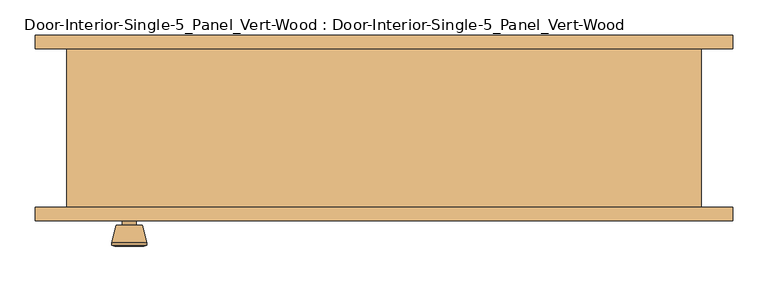
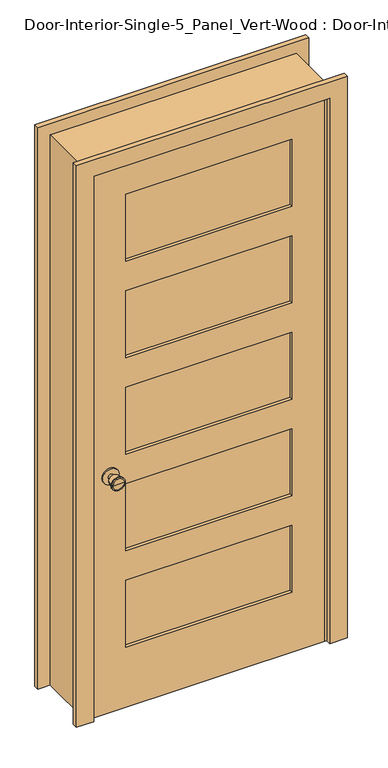
"""IFC4 building model written with IfcOpenShell, lengths in millimetres: door geometry, Door-Interior-Single-5_Panel_Vert-Wood : Door-Interior-Single-5_Panel_Vert-Wood."""

from ifc_helpers import new_model, si_unit, point, frame, frame_2d, origin, place, context, project, spatial, polyline, circle_curve, trimmed, segment, composite_curve, outline, extrude, faceted_brep, source, transform, mapped, element, save
from ifc_brep_helpers import plane_surface, cylinder_surface, revolved_surface, advanced_brep


def door_interior_single_5_panel_vert_wood_door_interior_single_643f6a0b(model_context):
    return source(origin(), model_context, "Body", "SolidModel", [
        advanced_brep(
        [(-361.1, -68.4, 914.4), (-371.1, -68.4, 914.4), (-351.1, -68.4, 914.4), (-340.6241324, -19.4, 914.4), (-381.5758676, -19.4, 914.4), (-361.1, -19.4, 914.4), (-336.1, -21.2278681, 914.4), (-386.1, -21.2278681, 914.4), (-336.1, -24.6915463, 914.4), (-386.1, -24.6915463, 914.4), (-342.463764, -49.4, 914.4), (-379.736236, -49.4, 914.4), (-351.1, -49.4, 914.4), (-371.1, -49.4, 914.4)],
        [
            (0, 1),
            (1, 2, circle_curve(frame((-361.1, -68.4, 914.4), z_axis=(0.0, -1.0, 0.0), x_axis=(-1.0, 0.0, 0.0)), 10.0)),
            (2, 0),
            (2, 1, circle_curve(frame((-361.1, -68.4, 914.4), z_axis=(0.0, -1.0, 0.0), x_axis=(-1.0, 0.0, 0.0)), 10.0)),
            (3, 4, circle_curve(frame((-361.1, -19.4, 914.4), z_axis=(0.0, 1.0, 0.0), x_axis=(-1.0, 0.0, 0.0)), 20.4758676)),
            (4, 5),
            (5, 3),
            (4, 3, circle_curve(frame((-361.1, -19.4, 914.4), z_axis=(0.0, 1.0, 0.0), x_axis=(-1.0, 0.0, 0.0)), 20.4758676)),
            (6, 7, circle_curve(frame((-361.1, -21.2278681, 914.4), z_axis=(0.0, 1.0, 0.0), x_axis=(-1.0, 0.0, 0.0)), 25.0)),
            (7, 4),
            (3, 6),
            (7, 6, circle_curve(frame((-361.1, -21.2278681, 914.4), z_axis=(0.0, 1.0, 0.0), x_axis=(-1.0, 0.0, 0.0)), 25.0)),
            (8, 9, circle_curve(frame((-361.1, -24.6915463, 914.4), z_axis=(0.0, 1.0, 0.0), x_axis=(-1.0, 0.0, 0.0)), 25.0)),
            (9, 7),
            (6, 8),
            (9, 8, circle_curve(frame((-361.1, -24.6915463, 914.4), z_axis=(0.0, 1.0, 0.0), x_axis=(-1.0, 0.0, 0.0)), 25.0)),
            (10, 11, circle_curve(frame((-361.1, -49.4, 914.4), z_axis=(0.0, 1.0, 0.0), x_axis=(-1.0, 0.0, 0.0)), 18.636236)),
            (11, 9),
            (8, 10),
            (11, 10, circle_curve(frame((-361.1, -49.4, 914.4), z_axis=(0.0, 1.0, 0.0), x_axis=(-1.0, 0.0, 0.0)), 18.636236)),
            (12, 13, circle_curve(frame((-361.1, -49.4, 914.4), z_axis=(0.0, 1.0, 0.0), x_axis=(-1.0, 0.0, 0.0)), 10.0)),
            (13, 11),
            (10, 12),
            (13, 12, circle_curve(frame((-361.1, -49.4, 914.4), z_axis=(0.0, 1.0, 0.0), x_axis=(-1.0, 0.0, 0.0)), 10.0)),
            (1, 13),
            (12, 2),
        ],
        [
            plane_surface(frame((-361.1, -68.4, 914.4), z_axis=(0.0, -1.0, 0.0), x_axis=(-1.0, 0.0, 0.0))),
            plane_surface(frame((-361.1, -19.4, 914.4), z_axis=(0.0, 1.0, 0.0), x_axis=(-1.0, 0.0, 0.0))),
            revolved_surface(polyline([(-381.5758676, -19.4, 914.4), (-386.1, -21.2278681, 914.4)]), (-361.1, -68.4, 914.4), (0.0, -1.0, 0.0)),
            cylinder_surface(frame((-361.1, -68.4, 914.4), z_axis=(0.0, -1.0, 0.0), x_axis=(-1.0, 0.0, 0.0)), 25.0),
            revolved_surface(polyline([(-386.1, -24.6915463, 914.4), (-379.736236, -49.4, 914.4)]), (-361.1, -68.4, 914.4), (0.0, -1.0, 0.0)),
            plane_surface(frame((-361.1, -49.4, 914.4), z_axis=(0.0, -1.0, 0.0), x_axis=(-1.0, 0.0, 0.0))),
            cylinder_surface(frame((-361.1, -68.4, 914.4), z_axis=(0.0, -1.0, 0.0), x_axis=(-1.0, 0.0, 0.0)), 10.0),
        ],
        [
            (0, [[1, 2, 3]]),
            (0, [[-3, 4, -1]]),
            (1, [[5, 6, 7]]),
            (1, [[8, -7, -6]]),
            (2, [[9, 10, -5, 11]]),
            (2, [[12, -11, -8, -10]]),
            (3, [[13, 14, -9, 15]]),
            (3, [[16, -15, -12, -14]]),
            (4, [[17, 18, -13, 19]]),
            (4, [[20, -19, -16, -18]]),
            (5, [[21, 22, -17, 23]]),
            (5, [[24, -23, -20, -22]]),
            (6, [[-2, 25, -21, 26]]),
            (6, [[-4, -26, -24, -25]]),
        ],
    ),
        extrude(outline(composite_curve([segment(trimmed(circle_curve(frame_2d((914.4, -361.1)), 30.0), [point((914.4, -391.1))], [point((914.4, -331.1))], False, "CARTESIAN"), True, "CONTINUOUS"), segment(trimmed(circle_curve(frame_2d((914.4, -361.1)), 30.0), [point((914.4, -331.1))], [point((914.4, -391.1))], False, "CARTESIAN"), True, "CONTINUOUS")], self_intersect=False)), frame((0.0, -74.4, 0.0), z_axis=(0.0, 1.0, 0.0), x_axis=(0.0, 0.0, 1.0)), (0.0, 0.0, 1.0), 6.0),
        advanced_brep(
        [(-361.1, -115.325, 914.4), (-351.1, -115.325, 914.4), (-371.1, -115.325, 914.4), (-340.6241324, -164.325, 914.4), (-361.1, -164.325, 914.4), (-381.5758676, -164.325, 914.4), (-336.1, -162.4971319, 914.4), (-386.1, -162.4971319, 914.4), (-336.1, -159.0334537, 914.4), (-386.1, -159.0334537, 914.4), (-342.463764, -134.325, 914.4), (-379.736236, -134.325, 914.4), (-351.1, -134.325, 914.4), (-371.1, -134.325, 914.4)],
        [
            (0, 1),
            (1, 2, circle_curve(frame((-361.1, -115.325, 914.4), z_axis=(0.0, 1.0, 0.0), x_axis=(-1.0, 0.0, 0.0)), 10.0)),
            (2, 0),
            (2, 1, circle_curve(frame((-361.1, -115.325, 914.4), z_axis=(0.0, 1.0, 0.0), x_axis=(-1.0, 0.0, 0.0)), 10.0)),
            (3, 4),
            (4, 5),
            (5, 3, circle_curve(frame((-361.1, -164.325, 914.4), z_axis=(0.0, -1.0, 0.0), x_axis=(-1.0, 0.0, 0.0)), 20.4758676)),
            (3, 5, circle_curve(frame((-361.1, -164.325, 914.4), z_axis=(0.0, -1.0, 0.0), x_axis=(-1.0, 0.0, 0.0)), 20.4758676)),
            (6, 3),
            (5, 7),
            (7, 6, circle_curve(frame((-361.1, -162.4971319, 914.4), z_axis=(0.0, -1.0, 0.0), x_axis=(-1.0, 0.0, 0.0)), 25.0)),
            (6, 7, circle_curve(frame((-361.1, -162.4971319, 914.4), z_axis=(0.0, -1.0, 0.0), x_axis=(-1.0, 0.0, 0.0)), 25.0)),
            (8, 6),
            (7, 9),
            (9, 8, circle_curve(frame((-361.1, -159.0334537, 914.4), z_axis=(0.0, -1.0, 0.0), x_axis=(-1.0, 0.0, 0.0)), 25.0)),
            (8, 9, circle_curve(frame((-361.1, -159.0334537, 914.4), z_axis=(0.0, -1.0, 0.0), x_axis=(-1.0, 0.0, 0.0)), 25.0)),
            (10, 8),
            (9, 11),
            (11, 10, circle_curve(frame((-361.1, -134.325, 914.4), z_axis=(0.0, -1.0, 0.0), x_axis=(-1.0, 0.0, 0.0)), 18.636236)),
            (10, 11, circle_curve(frame((-361.1, -134.325, 914.4), z_axis=(0.0, -1.0, 0.0), x_axis=(-1.0, 0.0, 0.0)), 18.636236)),
            (12, 10),
            (11, 13),
            (13, 12, circle_curve(frame((-361.1, -134.325, 914.4), z_axis=(0.0, -1.0, 0.0), x_axis=(-1.0, 0.0, 0.0)), 10.0)),
            (12, 13, circle_curve(frame((-361.1, -134.325, 914.4), z_axis=(0.0, -1.0, 0.0), x_axis=(-1.0, 0.0, 0.0)), 10.0)),
            (1, 12),
            (13, 2),
        ],
        [
            plane_surface(frame((-361.1, -115.325, 914.4), z_axis=(0.0, 1.0, 0.0), x_axis=(-1.0, 0.0, 0.0))),
            plane_surface(frame((-361.1, -164.325, 914.4), z_axis=(0.0, -1.0, 0.0), x_axis=(-1.0, 0.0, 0.0))),
            revolved_surface(polyline([(-381.5758676, -164.325, 914.4), (-386.1, -162.4971319, 914.4)]), (-361.1, -115.325, 914.4), (0.0, 1.0, 0.0)),
            cylinder_surface(frame((-361.1, -115.325, 914.4), z_axis=(0.0, 1.0, 0.0), x_axis=(-1.0, 0.0, 0.0)), 25.0),
            revolved_surface(polyline([(-386.1, -159.0334537, 914.4), (-379.736236, -134.325, 914.4)]), (-361.1, -115.325, 914.4), (0.0, 1.0, 0.0)),
            plane_surface(frame((-361.1, -134.325, 914.4), z_axis=(0.0, 1.0, 0.0), x_axis=(-1.0, 0.0, 0.0))),
            cylinder_surface(frame((-361.1, -115.325, 914.4), z_axis=(0.0, 1.0, 0.0), x_axis=(-1.0, 0.0, 0.0)), 10.0),
        ],
        [
            (0, [[1, 2, 3]]),
            (0, [[-3, 4, -1]]),
            (1, [[5, 6, 7]]),
            (1, [[-6, -5, 8]]),
            (2, [[9, -7, 10, 11]]),
            (2, [[-10, -8, -9, 12]]),
            (3, [[13, -11, 14, 15]]),
            (3, [[-14, -12, -13, 16]]),
            (4, [[17, -15, 18, 19]]),
            (4, [[-18, -16, -17, 20]]),
            (5, [[21, -19, 22, 23]]),
            (5, [[-22, -20, -21, 24]]),
            (6, [[25, -23, 26, -2]]),
            (6, [[-26, -24, -25, -4]]),
        ],
    ),
        extrude(outline(composite_curve([segment(trimmed(circle_curve(frame_2d((914.4, -361.1)), 30.0), [point((914.4, -391.1))], [point((914.4, -331.1))], False, "CARTESIAN"), True, "CONTINUOUS"), segment(trimmed(circle_curve(frame_2d((914.4, -361.1)), 30.0), [point((914.4, -331.1))], [point((914.4, -391.1))], False, "CARTESIAN"), True, "CONTINUOUS")], self_intersect=False)), frame((0.0, -115.325, 0.0), z_axis=(0.0, 1.0, 0.0), x_axis=(0.0, 0.0, 1.0)), (0.0, 0.0, 1.0), 6.0),
        faceted_brep([(450.0, -109.325, 0.0), (424.6, -109.325, 0.0), (424.6, -74.4, 0.0), (411.9, -74.4, 0.0), (411.9, -39.475, 0.0), (424.6, -39.475, 0.0), (424.6, 115.675, 0.0), (450.0, 115.675, 0.0), (450.0, 115.675, 2125.4), (450.0, -109.325, 2125.4), (424.6, 115.675, 2100.0), (-424.6, 115.675, 2100.0), (-424.6, 115.675, 0.0), (-450.0, 115.675, 0.0), (-450.0, 115.675, 2125.4), (424.6, -39.475, 2100.0), (411.9, -39.475, 2087.3), (-411.9, -39.475, 2087.3), (-411.9, -39.475, 0.0), (-424.6, -39.475, 0.0), (-424.6, -39.475, 2100.0), (411.9, -74.4, 2087.3), (424.6, -74.4, 2100.0), (-424.6, -74.4, 2100.0), (-424.6, -74.4, 0.0), (-411.9, -74.4, 0.0), (-411.9, -74.4, 2087.3), (424.6, -109.325, 2100.0), (-450.0, -109.325, 2125.4), (-450.0, -109.325, 0.0), (-424.6, -109.325, 0.0), (-424.6, -109.325, 2100.0)], [[[0, 1, 2, 3, 4, 5, 6, 7]], [[7, 8, 9, 0]], [[6, 10, 11, 12, 13, 14, 8, 7]], [[5, 15, 10, 6]], [[4, 16, 17, 18, 19, 20, 15, 5]], [[3, 21, 16, 4]], [[2, 22, 23, 24, 25, 26, 21, 3]], [[1, 27, 22, 2]], [[0, 9, 28, 29, 30, 31, 27, 1]], [[8, 14, 28, 9]], [[15, 20, 11, 10]], [[21, 26, 17, 16]], [[27, 31, 23, 22]], [[29, 13, 12, 19, 18, 25, 24, 30]], [[14, 13, 29, 28]], [[20, 19, 12, 11]], [[26, 25, 18, 17]], [[31, 30, 24, 23]]]),
        extrude(outline(polyline([(2100.0, -424.6), (0.0, -424.6), (0.0, 424.6), (2100.0, 424.6), (2100.0, -424.6)]), holes=[polyline([(1980.9375, -303.95), (1980.9375, 303.95), (1722.545, 303.95), (1722.545, -303.95), (1980.9375, -303.95)]), polyline([(490.1675, -303.95), (490.1675, 303.95), (231.775, 303.95), (231.775, -303.95), (490.1675, -303.95)]), polyline([(1235.5525, -303.95), (1235.5525, 303.95), (977.16, 303.95), (977.16, -303.95), (1235.5525, -303.95)]), polyline([(1608.245, -303.95), (1608.245, 303.95), (1349.8525, 303.95), (1349.8525, -303.95), (1608.245, -303.95)]), polyline([(862.86, -303.95), (862.86, 303.95), (604.4675, 303.95), (604.4675, -303.95), (862.86, -303.95)])]), frame((0.0, -109.325, 0.0), z_axis=(0.0, 1.0, 0.0), x_axis=(0.0, 0.0, 1.0)), (0.0, 0.0, 1.0), 34.925),
        extrude(outline(polyline([(303.95, -86.0416667), (303.95, -97.6833333), (-303.95, -97.6833333), (-303.95, -86.0416667), (303.95, -86.0416667)])), frame((0.0, 0.0, 1722.545), z_axis=(0.0, 0.0, 1.0), x_axis=(1.0, 0.0, 0.0)), (0.0, 0.0, 1.0), 258.3925),
        extrude(outline(polyline([(303.95, -86.0416667), (303.95, -97.6833333), (-303.95, -97.6833333), (-303.95, -86.0416667), (303.95, -86.0416667)])), frame((0.0, 0.0, 1349.8525), z_axis=(0.0, 0.0, 1.0), x_axis=(1.0, 0.0, 0.0)), (0.0, 0.0, 1.0), 258.3925),
        extrude(outline(polyline([(303.95, -86.0416667), (303.95, -97.6833333), (-303.95, -97.6833333), (-303.95, -86.0416667), (303.95, -86.0416667)])), frame((0.0, 0.0, 604.4675), z_axis=(0.0, 0.0, 1.0), x_axis=(1.0, 0.0, 0.0)), (0.0, 0.0, 1.0), 258.3925),
        extrude(outline(polyline([(303.95, -86.0416667), (303.95, -97.6833333), (-303.95, -97.6833333), (-303.95, -86.0416667), (303.95, -86.0416667)])), frame((0.0, 0.0, 231.775), z_axis=(0.0, 0.0, 1.0), x_axis=(1.0, 0.0, 0.0)), (0.0, 0.0, 1.0), 258.3925),
        extrude(outline(polyline([(303.95, -86.0416667), (303.95, -97.6833333), (-303.95, -97.6833333), (-303.95, -86.0416667), (303.95, -86.0416667)])), frame((0.0, 0.0, 977.16), z_axis=(0.0, 0.0, 1.0), x_axis=(1.0, 0.0, 0.0)), (0.0, 0.0, 1.0), 258.3925),
        extrude(outline(polyline([(0.0, 494.45), (2169.85, 494.45), (2169.85, -494.45), (0.0, -494.45), (0.0, -430.95), (2106.35, -430.95), (2106.35, 430.95), (0.0, 430.95), (0.0, 494.45)])), frame((0.0, -128.375, 0.0), z_axis=(0.0, 1.0, 0.0), x_axis=(0.0, 0.0, 1.0)), (0.0, 0.0, 1.0), 19.05),
        extrude(outline(polyline([(0.0, 494.45), (2169.85, 494.45), (2169.85, -494.45), (0.0, -494.45), (0.0, -430.95), (2106.35, -430.95), (2106.35, 430.95), (0.0, 430.95), (0.0, 494.45)])), frame((0.0, 115.675, 0.0), z_axis=(0.0, 1.0, 0.0), x_axis=(0.0, 0.0, 1.0)), (0.0, 0.0, 1.0), 19.05),
    ])


if __name__ == "__main__":
    model = new_model("IFC4")
    model_context = context("Model", 3, world=origin())
    ifc_project = project(units=[si_unit("LENGTHUNIT", "METRE", prefix="MILLI")], contexts=[model_context])
    site = spatial("IfcSite", under=ifc_project)
    building = spatial("IfcBuilding", under=site)
    placement = place(None, origin())
    door_interior_single_5_panel_vert_wood_door_interior_single_shape = door_interior_single_5_panel_vert_wood_door_interior_single_643f6a0b(model_context)
    element("IfcDoor", 1, ObjectType="Door-Interior-Single-5_Panel_Vert-Wood : Door-Interior-Single-5_Panel_Vert-Wood", at=placement, inside=building, context=model_context, shape_type="MappedRepresentation", body=[
        mapped(door_interior_single_5_panel_vert_wood_door_interior_single_shape, transform((0.0, 0.0, 0.0), x_axis=(1.0, 0.0, 0.0), y_axis=(0.0, 1.0, 0.0), z_axis=(0.0, 0.0, 1.0))),
    ])
    save(model, "model.ifc")

# Revit data of these elements
# Type "Door-Interior-Single-5_Panel_Vert-Wood : Door-Interior-Single-5_Panel_Vert-Wood"
#   Type Mark = "46"
#   Assembly Code = "C1020300"
#   Analytic Construction = "Wooden"
#   Top Rail = 119.063 mm
#   Thickness = 34.925 mm
#   Thermal Resistance (R) = 0.455703 (m²·K)/W
#   Swing Angle [instance default] = 90.00°
#   Stiles = 120.65 mm
#   Rough Width = 900 mm
#   Rough Height = 2125.4 mm
#   Intermediate Rail = 114.3 mm
#   Height = 2100 mm
#   Width = 849.2 mm
#   Heat Transfer Coefficient (U) = 2.19465 W/(m²·K)
#   Bottom Rail = 231.775 mm
#   Trim Material = Cherry
#   Panel Material = Cherry
#   Frame Material = Cherry
#   Door Handle Material = Aluminum
#   Visual Light Transmittance = 0
#   Solar Heat Gain Coefficient = 0
#   Wall Closure = (empty or 0)
#   Function = (empty or 0)
# Element 1 (IfcDoor, "Door-Interior-Single-5_Panel_Vert-Wood : Door-Interior-Single-5_Panel_Vert-Wood")
#   Materials on its faces: "Cherry", "Aluminum"
# Materials
#   "Cherry": class "Wood", colour RGB 226 177 128, transparency 0, Description = "Prunus Serotina", Cost = 0
#   "Aluminum": class "Metal", colour RGB 247 247 247, transparency 0, Description = "Aluminum 6061", Cost = 0
